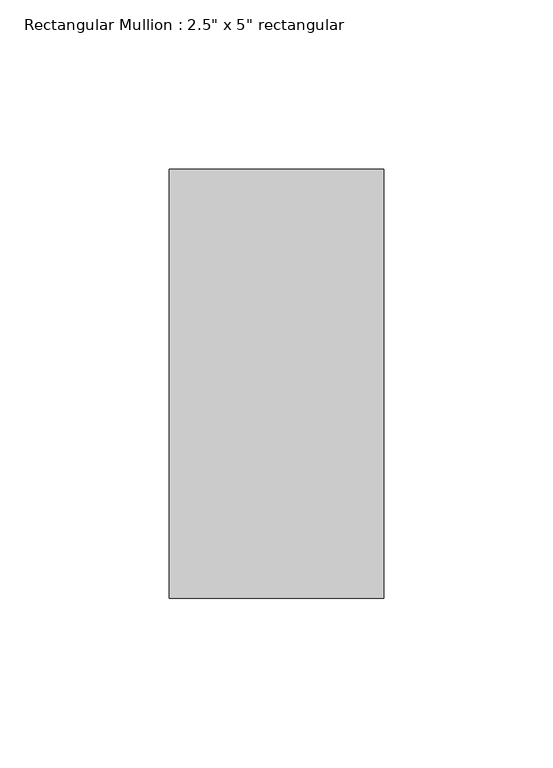
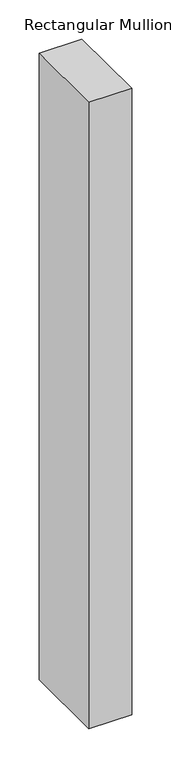
"""IFC4 building model written with IfcOpenShell, lengths in millimetres: member geometry."""

from ifc_helpers import new_model, si_unit, frame, origin, place, context, project, spatial, polyline, outline, extrude, source, transform, mapped, element, save


def member_19666b72(model_context):
    return source(origin(), model_context, "Body", "SweptSolid", [
        extrude(outline(polyline([(31.75, 63.5), (31.75, -63.5), (-31.75, -63.5), (-31.75, 63.5), (31.75, 63.5)])), frame((0.0, 0.0, -979.7309713), z_axis=(0.0, 0.0, 1.0), x_axis=(1.0, 0.0, 0.0)), (0.0, 0.0, 1.0), 979.7309713),
    ])


if __name__ == "__main__":
    model = new_model("IFC4")
    model_context = context("Model", 3, world=origin())
    ifc_project = project(units=[si_unit("LENGTHUNIT", "METRE", prefix="MILLI")], contexts=[model_context])
    site = spatial("IfcSite", under=ifc_project)
    building = spatial("IfcBuilding", under=site)
    placement = place(None, origin())
    member_shape = member_19666b72(model_context)
    element("IfcMember", 1, ObjectType="Rectangular Mullion : 2.5\" x 5\" rectangular", at=placement, inside=building, context=model_context, shape_type="MappedRepresentation", body=[
        mapped(member_shape, transform((0.0, 0.0, 0.0), x_axis=(1.0, 0.0, 0.0), y_axis=(0.0, 1.0, 0.0), z_axis=(0.0, 0.0, 1.0))),
    ])
    save(model, "model.ifc")

# Revit data of these elements
# Type "Rectangular Mullion : 2.5\" x 5\" rectangular"
#   built-in parameter 1007304 = 0.416667 (stored number, unit not read)
#   built-in parameter 1007301 = 0.104167 (stored number, unit not read)
#   built-in parameter 1007300 = 0.104167 (stored number, unit not read)
# Element 1 (IfcMember, "Rectangular Mullion : 2.5\" x 5\" rectangular")
#   Materials on its faces: "Aluminum"
# Materials
#   "Aluminum": class "Metal", colour RGB 247 247 247, transparency 0, Description = "Aluminum 6061", Cost = 0
